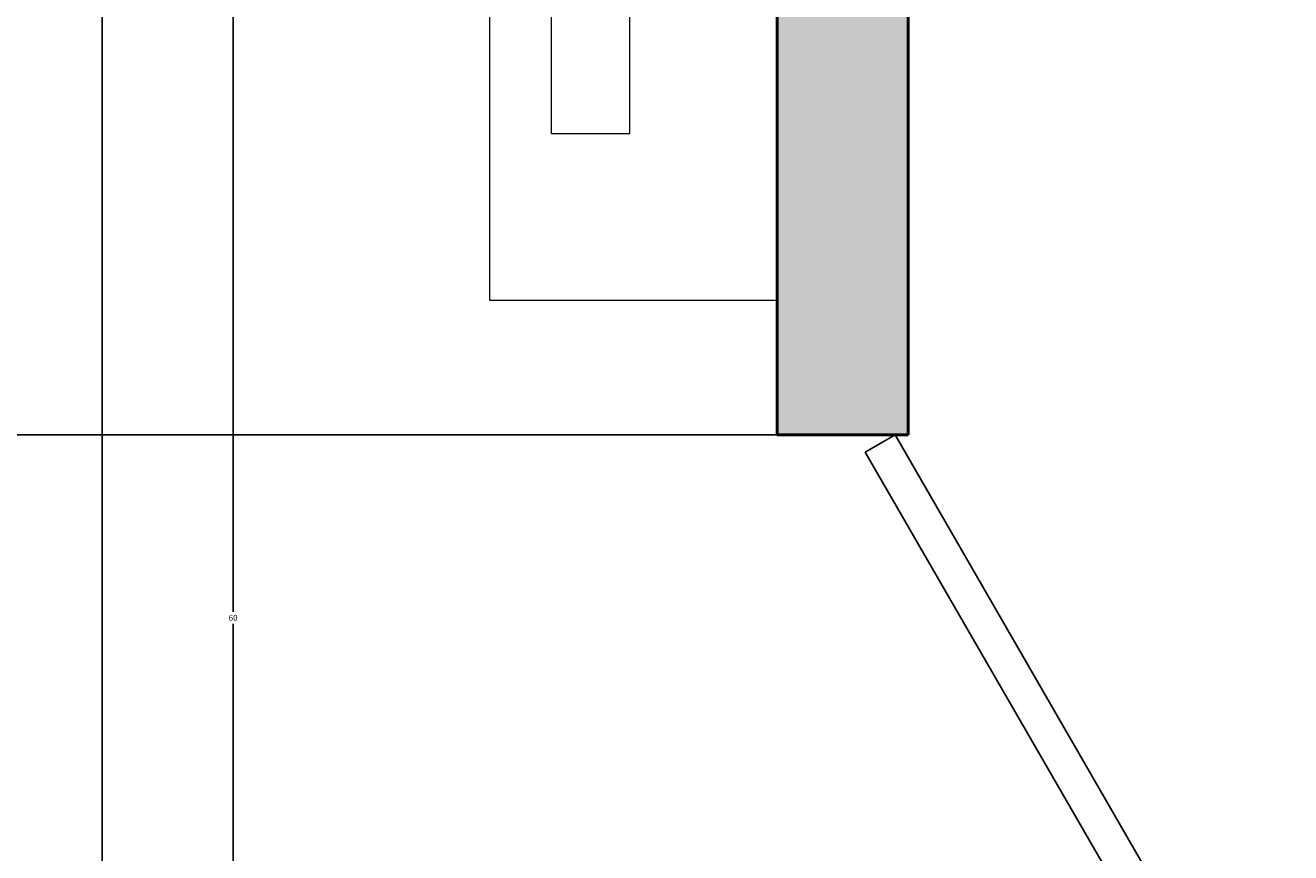
# Model space of a CAD drawing. Units: inches. Extents: x 2231 to 2461, y 2045 to 2455.
# Tile 80 of 95: x 2346 to 2384, y 2358 to 2383. Entities that reach past the tile are written whole.
import ezdxf

# ---------------------------------------------------------------- set-up
doc = ezdxf.new("R2010")
doc.units = ezdxf.units.IN
for name, color, linetype, lineweight in [('A-ANNO-DIMS', 2, 'Continuous', 18), ('A-DOOR', 3, 'Continuous', 25), ('A-EQPM', 8, 'Continuous', 18), ('A-FURN', 9, 'Continuous', 18), ('A-WALL', 7, 'Continuous', 50)]:
    doc.layers.add(name, color=color, linetype=linetype, lineweight=lineweight)
doc.layers.add('A-WALL-PATT', color=18, linetype='Continuous', lineweight=13, true_color=0x000000)
doc.styles.get("Standard").update_dxf_attribs({"font": 'arial.ttf'})
doc.dimstyles.get("Standard").update_dxf_attribs({"dimtxt": 0.18, "dimasz": 0.18, "dimexe": 0.18, "dimexo": 0.0625, "dimgap": 0.09, "dimtad": 0, "dimtih": 1, "dimtoh": 1, "dimdec": 4, "dimzin": 0, "dimdsep": 46, "dimtxsty": 'Standard', "dimcen": 0.09, "dimadec": 0, "dimazin": 0, "dimtfac": 1, "dimtdec": 4, "dimtofl": 0, "dimtmove": 0, "dimatfit": 3, "dimfxl": 1, "dimtolj": 1, "dimtzin": 0, "dimarcsym": 0})

# ---------------------------------------------------------------- blocks, each defined once
blk = doc.blocks.new('*U3')
for p, q in [((0, 0), (0, -6)), ((40, 0), (40, -6))]:
    blk.add_line(p, q)
blk.add_lwpolyline([(0, 0), (34.641, 20), (35.516, 18.484), (0.875, -1.516)], close=True)
blk.add_arc((0, 0), 40, 0, 30)
blk = doc.blocks.new('*D20')
at = {"layer": 'A-ANNO-DIMS', "color": 0, "lineweight": -2, "transparency": 16777216}
for p, q in [((2340.251, 2395.253), (2352.368, 2395.253)), ((2352.188, 2395.073), (2352.188, 2365.435)), ((2352.188, 2335.433), (2352.188, 2365.071)), ((2340.251, 2335.253), (2352.368, 2335.253))]:
    blk.add_line(p, q, dxfattribs=at)
at = {"layer": 'A-ANNO-DIMS', "color": 0, "transparency": 16777216}
for points in [[(2352.158, 2395.073), (2352.218, 2395.073), (2352.188, 2395.253)], [(2352.158, 2335.433), (2352.218, 2335.433), (2352.188, 2335.253)]]:
    blk.add_solid(points, dxfattribs=at)
at = {"layer": 'Defpoints', "color": 0, "transparency": 16777216}
for p in [(2340.188, 2395.253), (2352.188, 2395.253), (2340.188, 2335.253)]:
    blk.add_point(p, dxfattribs=at)
at = {"layer": 'A-ANNO-DIMS', "color": 0, "transparency": 16777216, "insert": (2352.188, 2365.253), "char_height": 0.18, "attachment_point": 5}
blk.add_mtext('\\A1;60', dxfattribs=at)
blk = doc.blocks.new('*D54')
at = {"layer": 'A-ANNO-DIMS', "color": 0, "lineweight": -2, "transparency": 16777216}
for p, q in [((2372.731, 2370.833), (2230.981, 2370.833)), ((2231.161, 2370.653), (2231.161, 2359.013)), ((2231.161, 2347.013), (2231.161, 2358.652)), ((2372.731, 2346.833), (2230.981, 2346.833))]:
    blk.add_line(p, q, dxfattribs=at)
at = {"layer": 'A-ANNO-DIMS', "color": 0, "transparency": 16777216}
for points in [[(2231.131, 2370.653), (2231.191, 2370.653), (2231.161, 2370.833)], [(2231.131, 2347.013), (2231.191, 2347.013), (2231.161, 2346.833)]]:
    blk.add_solid(points, dxfattribs=at)
at = {"layer": 'Defpoints', "color": 0, "transparency": 16777216}
for p in [(2231.161, 2370.833), (2372.794, 2370.833), (2372.794, 2346.833)]:
    blk.add_point(p, dxfattribs=at)
at = {"layer": 'A-ANNO-DIMS', "color": 0, "transparency": 16777216, "insert": (2231.161, 2358.833), "char_height": 0.18, "attachment_point": 5}
blk.add_mtext('\\A1;24', dxfattribs=at)
blk = doc.blocks.new('*D66')
at = {"layer": 'A-ANNO-DIMS', "color": 0, "lineweight": -2, "transparency": 16777216}
for p, q in [((2348.189, 2096.895), (2348.189, 2454.645)), ((2408.794, 2096.895), (2408.794, 2454.645)), ((2348.369, 2454.465), (2378.167, 2454.465)), ((2408.614, 2454.465), (2378.815, 2454.465))]:
    blk.add_line(p, q, dxfattribs=at)
at = {"layer": 'A-ANNO-DIMS', "color": 0, "transparency": 16777216}
for points in [[(2348.369, 2454.495), (2348.369, 2454.435), (2348.189, 2454.465)], [(2408.614, 2454.495), (2408.614, 2454.435), (2408.794, 2454.465)]]:
    blk.add_solid(points, dxfattribs=at)
at = {"layer": 'Defpoints', "color": 0, "transparency": 16777216}
for p in [(2408.794, 2454.465), (2348.189, 2096.833), (2408.794, 2096.833)]:
    blk.add_point(p, dxfattribs=at)
at = {"layer": 'A-ANNO-DIMS', "color": 0, "transparency": 16777216, "insert": (2378.491, 2454.465), "char_height": 0.18, "attachment_point": 5}
blk.add_mtext('\\A1;60.6', dxfattribs=at)

msp = doc.modelspace()

# ---------------------------------------------------------------- hatches: boundary and pattern name
at = {"layer": 'A-WALL-PATT'}
h = msp.add_hatch(color=256, dxfattribs=at)
h.dxf.hatch_style = 1
h.paths.add_polyline_path([(2441.7935, 2269.1535), (2432.7935, 2269.1535), (2432.7935, 2186.8328), (2396.7935, 2186.8328), (2396.7935, 2286.8328), (2394.7935, 2286.8328), (2394.7935, 2186.8328), (2334.7935, 2186.8328), (2334.7935, 2182.8328), (2432.7935, 2182.8328), (2432.7935, 2072.8328), (2416.6639, 2072.8328), (2416.6639, 2063.8328), (2441.7935, 2063.8328)])
h.paths.add_polyline_path([(2368.6639, 2072.8328), (2367.04, 2072.8328), (2330.7942, 2072.8328), (2330.7397, 2063.8328), (2368.6639, 2063.8328)])
h.paths.add_polyline_path([(2300.7392, 2068.3328), (2300.7392, 2072.8328), (2298.7935, 2072.8328), (2294.7935, 2072.8328), (2258.7935, 2072.8328), (2258.7935, 2120.8328), (2294.7935, 2120.8328), (2298.7935, 2120.8328), (2298.7935, 2128.8328), (2294.7935, 2128.8328), (2294.7935, 2124.8328), (2258.7935, 2124.8328), (2258.7935, 2182.8328), (2294.7935, 2182.8328), (2294.7935, 2174.8328), (2298.7935, 2174.8328), (2298.7935, 2182.8328), (2304.7935, 2182.8328), (2304.7935, 2186.8328), (2258.7935, 2186.8328), (2258.7935, 2221.999), (2249.7935, 2221.999), (2249.7935, 2063.8328), (2300.7392, 2063.8328)])
h.paths.add_polyline_path([(2391.9338, 2435.8328), (2333.82, 2435.8328), (2333.82, 2426.8328), (2368.7935, 2426.8328), (2368.7935, 2374.9508), (2368.7935, 2370.8328), (2372.3935, 2370.8328), (2372.7935, 2370.8328), (2372.7935, 2426.8328), (2391.9338, 2426.8328)])
h.paths.add_polyline_path([(2441.7935, 2435.8328), (2415.9338, 2435.8328), (2415.9338, 2426.8328), (2432.7935, 2426.8328), (2432.7935, 2334.8328), (2372.7935, 2334.8328), (2372.7935, 2346.8328), (2368.7935, 2346.8328), (2368.7935, 2306.8328), (2360.7935, 2306.8328), (2360.7935, 2302.8328), (2368.7935, 2302.8328), (2372.7935, 2302.8328), (2372.7935, 2330.8328), (2432.7935, 2330.8328), (2432.7935, 2317.1535), (2441.7935, 2317.1535)])
h.paths.add_polyline_path([(2285.82, 2435.8328), (2249.7935, 2435.8328), (2249.7935, 2269.999), (2258.7935, 2269.999), (2258.7935, 2302.8328), (2318.8168, 2302.8328), (2330.7935, 2302.8328), (2330.7935, 2306.8328), (2258.7935, 2306.8328), (2258.7935, 2426.8328), (2285.82, 2426.8328)])

# ---------------------------------------------------------------- linework, layer by layer
at = {"layer": 'A-EQPM'}
msp.add_lwpolyline([(2361.91, 2421.8956), (2364.2888, 2421.8956), (2364.2888, 2380.0244), (2361.91, 2380.0244)], close=True, dxfattribs=at)
at = {"layer": 'A-FURN'}
msp.add_lwpolyline([(2368.7935, 2426.8328), (2360.0091, 2426.8328), (2360.0091, 2374.9508), (2368.7935, 2374.9508)], close=True, dxfattribs=at)
at = {"layer": 'A-WALL'}
for p, q in [((2368.7935, 2426.8328), (2368.7935, 2370.8328)), ((2372.7935, 2426.8328), (2372.7935, 2370.8328)), ((2372.7935, 2370.8328), (2368.7935, 2370.8328))]:
    msp.add_line(p, q, dxfattribs=at)

# ---------------------------------------------------------------- block references
at = {"layer": 'A-DOOR', "xscale": 0.6, "yscale": 0.6, "zscale": 0.6, "rotation": 270}
msp.add_blockref('*U3', (2372.3935, 2370.8328), dxfattribs=at)

# ---------------------------------------------------------------- dimensions: what is measured, and where the dimension line sits
at = {"layer": 'A-ANNO-DIMS'}
dim = msp.add_linear_dim(base=(2408.7935, 2454.4653), p1=(2348.1888, 2096.8328), p2=(2408.7935, 2096.8328), dimstyle='Standard', override={"dimdec": 1, "dimlfac": 1, "dimrnd": 0, "dimzin": 0, "dimdsep": 46, "dimlunit": 2}, dxfattribs=at)
dim.commit()
dim.dimension.update_dxf_attribs({"geometry": '*D66', "text_midpoint": (2378.4912, 2454.4653)})
for base, p1, p2, picture, middle in [((2352.1882, 2395.2534), (2340.1882, 2335.2534), (2340.1882, 2395.2534), '*D20', (2352.1882, 2365.2534)), ((2231.161, 2370.8328), (2372.7935, 2346.8328), (2372.7935, 2370.8328), '*D54', (2231.161, 2358.8328))]:
    dim = msp.add_linear_dim(base=base, p1=p1, p2=p2, angle=90, dimstyle='Standard', override={"dimdec": 0, "dimlfac": 1, "dimrnd": 0, "dimzin": 0, "dimdsep": 46, "dimlunit": 2}, dxfattribs=at)
    dim.commit()
    dim.dimension.update_dxf_attribs({"geometry": picture, "text_midpoint": middle})

doc.saveas('drawing.dxf')
